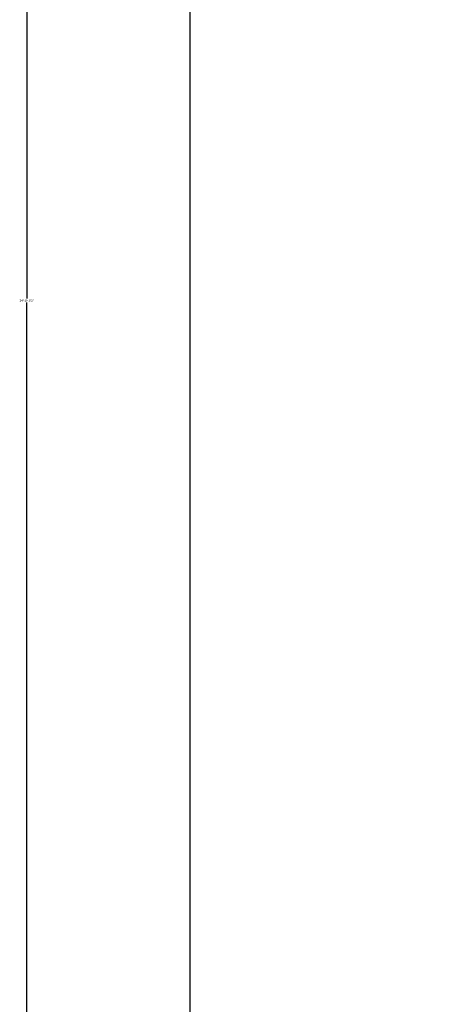
# Model space of a CAD drawing. Units: inches. Extents: x -9 to 505, y -680 to 48.
# Tile 8 of 17: x -9 to 27, y -198 to -114. Entities that reach past the tile are written whole.
import ezdxf

# ---------------------------------------------------------------- set-up
doc = ezdxf.new("R2010")
doc.units = ezdxf.units.IN
doc.header["$MEASUREMENT"] = 0
doc.layers.add('A-ANNO-DIMS', color=2, linetype='Continuous', lineweight=18)
doc.styles.get("Standard").update_dxf_attribs({"font": 'arial.ttf'})
doc.dimstyles.get("Standard").update_dxf_attribs({"dimtxt": 0.18, "dimasz": 0.18, "dimexe": 0.18, "dimexo": 0.0625, "dimgap": 0.09, "dimtad": 0, "dimtih": 1, "dimtoh": 1, "dimdec": 0, "dimzin": 0, "dimdsep": 46, "dimlunit": 3, "dimtxsty": 'Standard', "dimcen": 0.09, "dimadec": 0, "dimazin": 0, "dimtfac": 1, "dimtdec": 0, "dimtofl": 0, "dimtmove": 0, "dimatfit": 3, "dimfxl": 1, "dimtolj": 1, "dimtzin": 0, "dimarcsym": 0})

# ---------------------------------------------------------------- blocks, each defined once
blk = doc.blocks.new('*D3')
at = {"layer": 'A-ANNO-DIMS', "color": 0, "lineweight": -2, "transparency": 16777216}
for p, q in [((27.201, 11.499), (5.161, 11.499)), ((5.341, 11.319), (5.341, -330.86)), ((5.341, -679.321), (5.341, -337.142)), ((27.201, -679.501), (5.161, -679.501))]:
    blk.add_line(p, q, dxfattribs=at)
at = {"layer": 'A-ANNO-DIMS', "color": 0, "transparency": 16777216}
for points in [[(5.311, 11.319), (5.371, 11.319), (5.341, 11.499)], [(5.311, -679.321), (5.371, -679.321), (5.341, -679.501)]]:
    blk.add_solid(points, dxfattribs=at)
at = {"layer": 'Defpoints', "color": 0, "transparency": 16777216}
for p in [(27.264, 11.499), (5.341, -679.501), (27.264, -679.501)]:
    blk.add_point(p, dxfattribs=at)
at = {"layer": 'A-ANNO-DIMS', "color": 0, "transparency": 16777216, "insert": (5.341, -334.001), "char_height": 6, "attachment_point": 5}
blk.add_mtext('\\A1;57\'-7"', dxfattribs=at)
blk = doc.blocks.new('*D46')
at = {"layer": 'A-ANNO-DIMS', "color": 0, "lineweight": -2, "transparency": 16777216}
for p, q in [((27.201, 11.499), (-8.796, 11.499)), ((-8.616, 11.319), (-8.616, -137.568)), ((-8.616, -286.821), (-8.616, -137.934)), ((27.201, -287.001), (-8.796, -287.001))]:
    blk.add_line(p, q, dxfattribs=at)
at = {"layer": 'A-ANNO-DIMS', "color": 0, "transparency": 16777216}
for points in [[(-8.646, 11.319), (-8.586, 11.319), (-8.616, 11.499)], [(-8.646, -286.821), (-8.586, -286.821), (-8.616, -287.001)]]:
    blk.add_solid(points, dxfattribs=at)
at = {"layer": 'Defpoints', "color": 0, "transparency": 16777216}
for p in [(27.264, 11.499), (-8.616, -287.001), (27.264, -287.001)]:
    blk.add_point(p, dxfattribs=at)
at = {"layer": 'A-ANNO-DIMS', "color": 0, "transparency": 16777216, "insert": (-8.616, -137.751), "char_height": 0.18, "attachment_point": 5}
blk.add_mtext('\\A1;24\'-10 1/2"', dxfattribs=at)

msp = doc.modelspace()

# ---------------------------------------------------------------- dimensions: what is measured, and where the dimension line sits
at = {"layer": 'A-ANNO-DIMS'}
for base, p2, override, picture, middle in [((-8.616, -287.001), (27.264, -287.001), {"dimdec": 1, "dimlfac": 1, "dimrnd": 0, "dimzin": 1, "dimdsep": 46, "dimlunit": 4, "dimfrac": 2}, '*D46', (-8.616, -137.751)), ((5.341, -679.501), (27.264, -679.501), {"dimtxt": 6, "dimclrd": 0, "dimclre": 0, "dimclrt": 0}, '*D3', (5.341, -334.001))]:
    dim = msp.add_linear_dim(base=base, p1=(27.264, 11.499), p2=p2, angle=90, dimstyle='Standard', override=override, dxfattribs=at)
    dim.commit()
    dim.dimension.update_dxf_attribs({"geometry": picture, "text_midpoint": middle})

doc.saveas('drawing.dxf')
